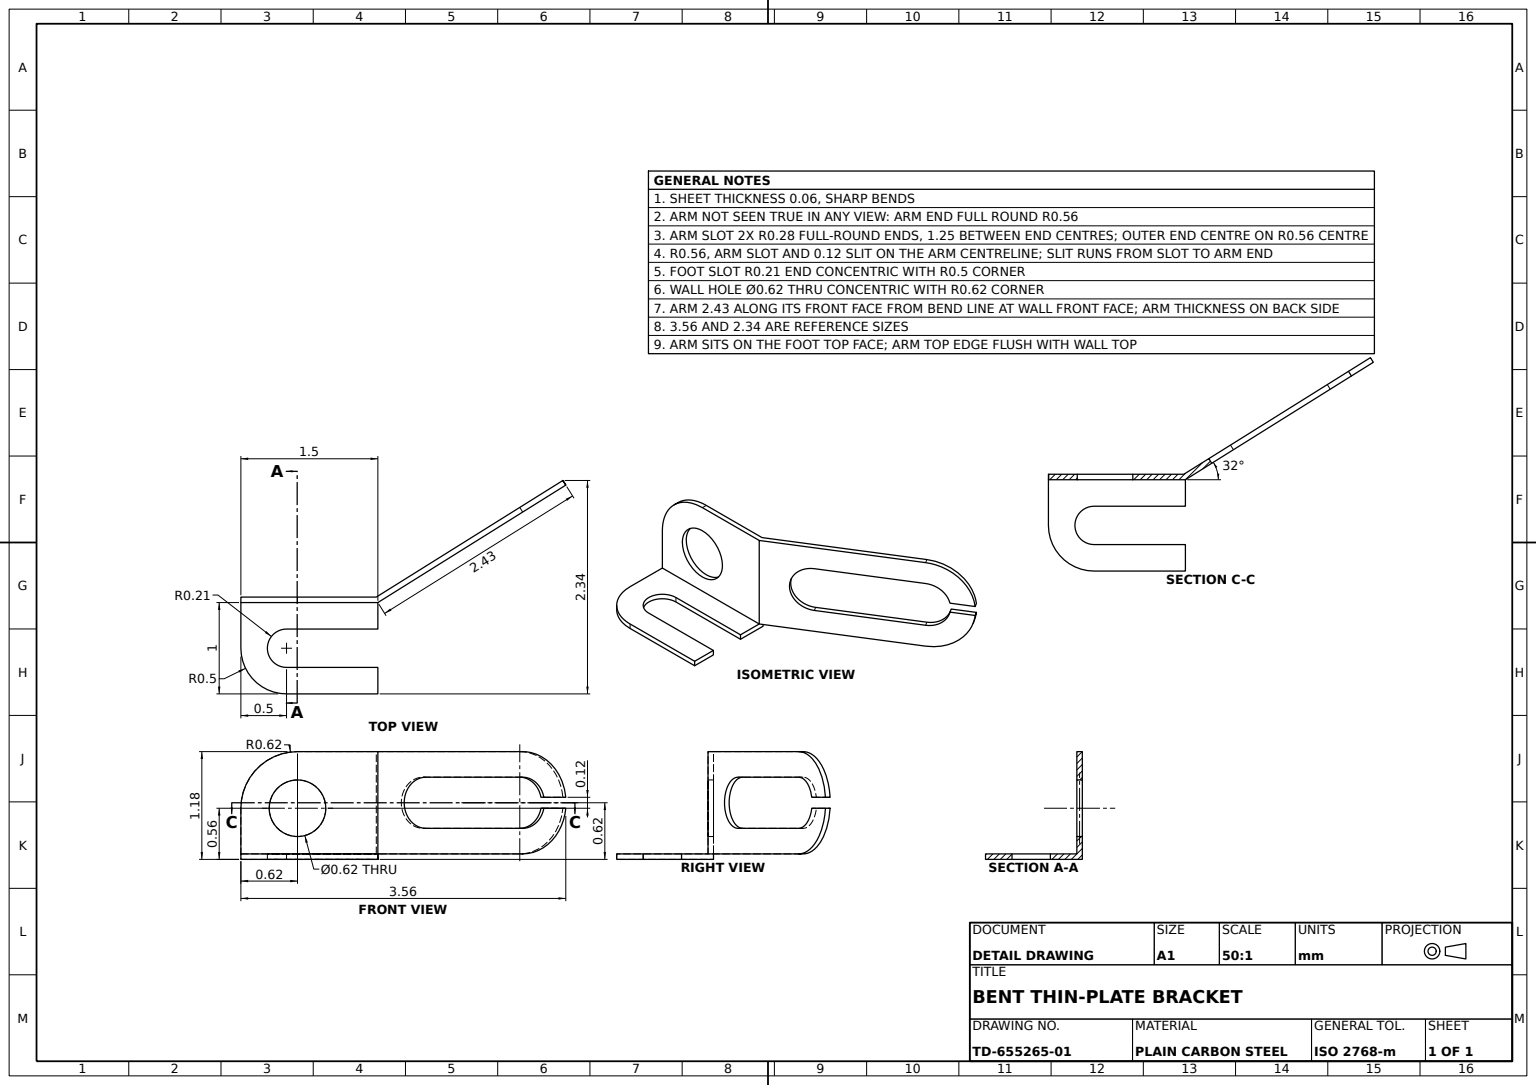
from build123d import *
from OCP.BRepFilletAPI import BRepFilletAPI_MakeFillet

# Parameters (mm, degrees)
VERTICAL_TAB_SKETCH_W    = 1.5
VERTICAL_TAB_SKETCH_H    = 1.18
VERTICAL_TAB_DEPTH       = 0.06
FOOT_SKETCH_W            = 1.5
FOOT_SKETCH_H            = 1
FOOT_DEPTH               = 0.06
ARM_SKETCH_W             = 2.43
ARM_SKETCH_H             = 1.12
ANGLED_ARM_DEPTH         = 0.06
TAB_CORNER_ROUNDS_R1     = 0.62
TAB_CORNER_ROUNDS_R2     = 0.5
TAB_HOLE_SKETCH_R        = 0.31
TAB_HOLE_DEPTH           = 0.06
FOOT_OPEN_SLOT_DEPTH     = 0.06
ARM_END_ROUNDS_RADIUS    = 0.56
ARM_END_ROUNDS_LENGTH    = 0.06
ARM_SLOT_WITH_SLIT_DEPTH = 0.06


with BuildPart() as part:
    # Vertical Tab Sketch → Vertical Tab (new body)
    with BuildSketch(Plane.XY):
        with Locations((-0.75, 0.53)):
            Rectangle(VERTICAL_TAB_SKETCH_W, VERTICAL_TAB_SKETCH_H)
    extrude(amount=-VERTICAL_TAB_DEPTH)

    # Foot Sketch → Foot (add)
    with BuildSketch(Plane(origin=(0, 0, 0), x_dir=(1, 0, 0), z_dir=(0, 1, 0))):
        with Locations((-0.75, -0.5)):
            Rectangle(FOOT_SKETCH_W, FOOT_SKETCH_H)
    extrude(amount=-FOOT_DEPTH)

    # Arm Sketch → Angled Arm (add)
    with BuildSketch(Plane(origin=(0, 0, 0), x_dir=(0.8480480961564255, 0, -0.5299192642332059), z_dir=(-0.5299192642332058, 0, -0.8480480961564254))):
        with Locations((1.215, -0.56)):
            Rectangle(ARM_SKETCH_W, ARM_SKETCH_H)
    extrude(amount=ANGLED_ARM_DEPTH)

    # Tab Corner Rounds: one fillet with a radius per group of edges: ONE call of the kernel's fillet builder (fillet() takes one radius for all edges)
    tab_corner_rounds_edges_1 = [part.edges().sort_by_distance(p)[0] for p in [
        (-1.5, 1.12, -0.03),
    ]]
    tab_corner_rounds_edges_2 = [part.edges().sort_by_distance(p)[0] for p in [
        (-1.5, -0.03, 1),
    ]]
    tab_corner_rounds = BRepFilletAPI_MakeFillet(part.part.solid().wrapped)
    for e in tab_corner_rounds_edges_1:
        tab_corner_rounds.Add(TAB_CORNER_ROUNDS_R1, e.wrapped)
    for e in tab_corner_rounds_edges_2:
        tab_corner_rounds.Add(TAB_CORNER_ROUNDS_R2, e.wrapped)
    add(Compound.cast(tab_corner_rounds.Shape()), mode=Mode.REPLACE)

    # Tab Hole Sketch → Tab Hole (cut)
    with BuildSketch(Plane.XY):
        with Locations((-0.88, 0.5)):
            Circle(TAB_HOLE_SKETCH_R)
    extrude(amount=-TAB_HOLE_DEPTH, mode=Mode.SUBTRACT)

    # Foot Slot Sketch → Foot Open Slot (cut)
    with BuildSketch(Plane(origin=(0, 0, 0), x_dir=(1, 0, 0), z_dir=(0, 1, 0))):
        with BuildLine():
            Line((-1, -0.29), (0.146073604, -0.29))
            ThreePointArc((0.146073604, -0.29), (0.356073604, -0.5), (0.146073604, -0.71))
            Line((0.146073604, -0.71), (-1, -0.71))
            ThreePointArc((-1, -0.71), (-1.21, -0.5), (-1, -0.29))
        make_face()
    extrude(amount=-FOOT_OPEN_SLOT_DEPTH, mode=Mode.SUBTRACT)

    # Arm End Rounds: full round fillet: the end face becomes a half cylinder, R = half its width
    arm_end_rounds_face = Plane((2.044859296, 0.56, -1.313145255), x_dir=(0.529919264233, 0, 0.848048096156), z_dir=(0.848048096156, 0, -0.529919264233))  # on the end face: x along it, z out of the body
    arm_end_rounds_slab = arm_end_rounds_face.offset(-ARM_END_ROUNDS_RADIUS / 2) * Box(ARM_END_ROUNDS_LENGTH, 2 * ARM_END_ROUNDS_RADIUS, ARM_END_ROUNDS_RADIUS, mode=Mode.PRIVATE)  # the body's end, R deep
    arm_end_rounds_round = Plane((1.569952362, 0.56, -1.016390467), x_dir=(0.848048096156, 0, -0.529919264233), z_dir=(0.529919264233, 0, 0.848048096156)) * Cylinder(ARM_END_ROUNDS_RADIUS, ARM_END_ROUNDS_LENGTH, mode=Mode.PRIVATE)  # its axis R under the face
    add(arm_end_rounds_slab - arm_end_rounds_round, mode=Mode.SUBTRACT)

    # Arm Slot Sketch → Arm Slot with Slit (cut)
    with BuildSketch(Plane(origin=(0, 0, 0), x_dir=(0.8480480961564255, 0, -0.5299192642332059), z_dir=(0.5299192642332058, 0, 0.8480480961564254))):
        with BuildLine():
            Line((1.87, 0.28), (0.62, 0.28))
            ThreePointArc((0.62, 0.28), (0.34, 0.56), (0.62, 0.84))
            Line((0.62, 0.84), (1.87, 0.84))
            ThreePointArc((1.87, 0.84), (2.045499288, 0.778174242), (2.143495887, 0.62))
            Line((2.143495887, 0.62), (2.426776436, 0.62))
            Line((2.426776436, 0.62), (2.426776436, 0.5))
            Line((2.426776436, 0.5), (2.143495887, 0.5))
            ThreePointArc((2.143495887, 0.5), (2.045499288, 0.341825758), (1.87, 0.28))
        make_face()
    extrude(amount=-ARM_SLOT_WITH_SLIT_DEPTH, mode=Mode.SUBTRACT)


with BuildPart() as arm_slot_with_slit_kept_piece:
    # of the separate pieces the step leaves, the one the design keeps (arm_slot_with_slit_pieces_kept)
    add(part.part.solids().sort_by_distance((-1.5, -0.06, 0.5))[0])


solid = arm_slot_with_slit_kept_piece.part
